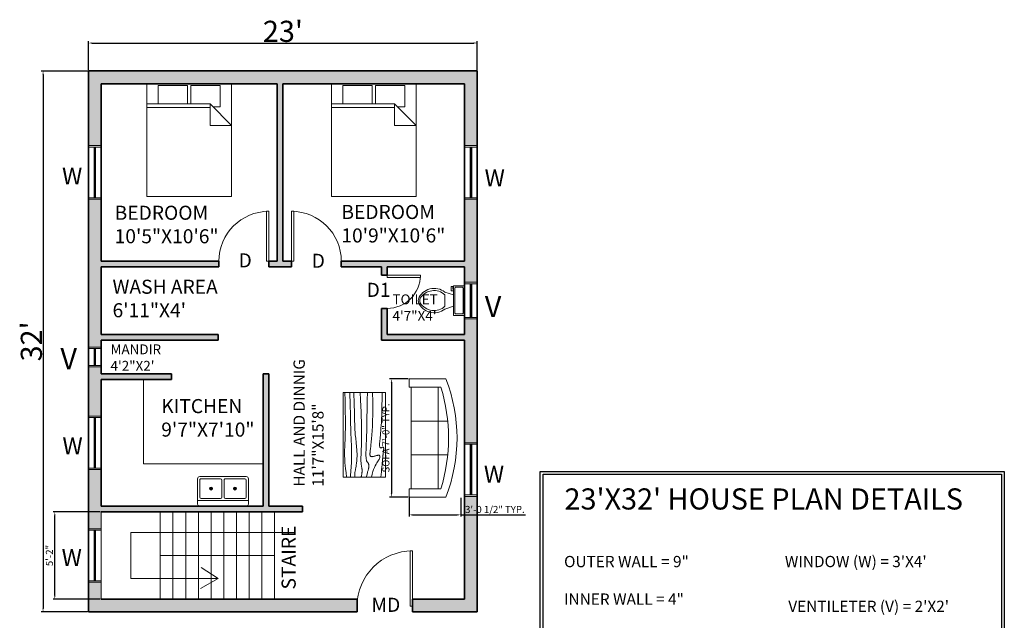
# Model space of a CAD drawing. Units: inches. Extents: x 1662 to 23131, y 1265 to 19127.
# Tile 7 of 26: x 12445 to 13143, y 5870 to 6296. Entities that reach past the tile are written whole.
import ezdxf

# ---------------------------------------------------------------- set-up
doc = ezdxf.new("R2010")
doc.units = ezdxf.units.IN
for name, color, linetype, lineweight in [('A-ANNO-DIMS', 4, 'Continuous', 18), ('A-ANNO-IDEN', 7, 'Continuous', 18), ('A-ANNO-TEXT', 7, 'Continuous', 18), ('A-ANNO-TITL', 7, 'Continuous', 35), ('A-ANNO-TTLB', 7, 'Continuous', 25), ('A-AREA-IDEN', 7, 'Continuous', 18), ('A-DOOR', 3, 'Continuous', 18), ('A-FLOR-CASE', 8, 'Continuous', 18), ('A-FLOR-FIXT', 9, 'Continuous', 18), ('A-FLOR-STRS', 7, 'Continuous', 18), ('A-FURN', 8, 'Continuous', 18), ('A-GLAZ', 4, 'Continuous', 18), ('A-WALL', 7, 'Continuous', 35), ('A-WALL-PATT', 8, 'Continuous', 13)]:
    doc.layers.add(name, color=color, linetype=linetype, lineweight=lineweight)
doc.styles.get("Standard").update_dxf_attribs({"font": 'arial.ttf'})
doc.dimstyles.new('ISO-25', dxfattribs={"dimtxt": 5, "dimasz": 2.5, "dimexe": 1.25, "dimexo": 0.625, "dimtad": 1, "dimlunit": 3, "dimtxsty": 'Standard', "dimcen": 2.5, "dimadec": 0, "dimazin": 0, "dimtfac": 1, "dimtmove": 0, "dimatfit": 3, "dimfxl": 1, "dimarcsym": 0})

# ---------------------------------------------------------------- blocks, each defined once
blk = doc.blocks.new('*U51')
for p, q in [((0, 0), (0, -100)), ((-1000, 0), (-1000, -100))]:
    blk.add_line(p, q)
blk.add_lwpolyline([(0, 0), (0, 1000), (-43.75, 1000), (-43.75, 0)], close=True)
blk.add_arc((0, 0), 1000, 90, 180)
blk = doc.blocks.new('*U26')
for p, q in [((0, 0), (0, -100)), ((900, 0), (900, -100))]:
    blk.add_line(p, q)
blk.add_lwpolyline([(0, 0), (0, 900), (43.75, 900), (43.75, 0)], close=True)
blk.add_arc((0, 0), 900, 0, 90)
blk = doc.blocks.new('*U4')
for p, q in [((0, 0), (0, -100)), ((-900, 0), (-900, -100))]:
    blk.add_line(p, q)
blk.add_lwpolyline([(0, 0), (0, 900), (-43.75, 900), (-43.75, 0)], close=True)
blk.add_arc((0, 0), 900, 90, 180)
blk = doc.blocks.new('*U28')
for p, q in [((0, 0), (0, -100)), ((600, 0), (600, -100))]:
    blk.add_line(p, q)
blk.add_lwpolyline([(0, 0), (0, 600), (43.75, 600), (43.75, 0)], close=True)
blk.add_arc((0, 0), 600, 0, 90)
blk = doc.blocks.new('Bed - Queen')
for p, q in [((0, -80.00003), (0, 0)), ((0, 0), (59.99999, 0)), ((59.99999, 0), (59.99999, -80.00003)), ((7.99999, -1.2), (28.79998, -1.2)), ((7.99999, -14.4), (7.99999, -1.2)), ((28.79998, -1.2), (28.79998, -14.4)), ((31.19999, -1.2), (51.99999, -1.2)), ((31.19999, -14.4), (31.19999, -1.2)), ((51.99999, -1.2), (51.99999, -16.4)), ((0, -14.4), (44.8, -14.4)), ((44.8, -16.8), (0, -16.8)), ((59.99999, -29.6), (44.8, -14.4)), ((44.8, -14.4), (44.8, -29.6)), ((51.99999, -16.4), (46.79936, -16.4)), ((44.8, -29.6), (59.99999, -29.6)), ((59.99999, -80.00003), (0, -80.00003))]:
    blk.add_line(p, q)
blk = doc.blocks.new('Sink-double - 36 in top')
for p, q in [((-18, -4), (18, -4)), ((-0.75, -18.5), (-0.75, -6.5)), ((0.75, -6.5), (0.75, -18.5))]:
    blk.add_line(p, q)
for points in [[(-16.5, 0), (16.5, 0)], [(-18, -19.5), (-18, -1.5)], [(-16.5, -18.5), (-16.5, -6.5)], [(-15.5, -5.5), (-1.75, -5.5)], [(1.75, -5.5), (15.5, -5.5)], [(16.5, -6.5), (16.5, -18.5)], [(18, -1.5), (18, -19.5)], [(-1.75, -19.5), (-15.5, -19.5)], [(15.5, -19.5), (1.75, -19.5)], [(16.5, -21), (-16.5, -21)]]:
    blk.add_lwpolyline(points)
for centre, radius in [((-8.5, -12.5), 1), ((-8.5, -12.5), 0.5), ((8.5, -12.5), 1), ((8.5, -12.5), 0.5)]:
    blk.add_circle(centre, radius)
for centre, radius, start, end in [((-16.5, -1.5), 1.5, 90, 180), ((16.5, -1.5), 1.5, 0, 90), ((-15.5, -6.5), 1, 90, 180), ((-1.75, -6.5), 1, 0, 90), ((1.75, -6.5), 1, 90, 180), ((15.5, -6.5), 1, 0, 90), ((-16.5, -19.5), 1.5, 180, 270), ((-15.5, -18.5), 1, 180, 270), ((-1.75, -18.5), 1, 270, 0), ((1.75, -18.5), 1, 180, 270), ((15.5, -18.5), 1, 270, 0), ((16.5, -19.5), 1.5, 270, 0)]:
    blk.add_arc(centre, radius, start, end)
blk = doc.blocks.new('Toilet - top')
for p, q in [((9.5, -6), (9.5, -2)), ((-10, -8.5), (-8, -8.5)), ((-10, -9.5), (-10, -8.5)), ((-7, -9.5), (-10, -9.5)), ((-8, -8.5), (-8, -8)), ((-7, -8), (-7, -9.5)), ((-4, -8), (-6, -14)), ((4, -8), (6, -14)), ((4, -14), (-4, -14))]:
    blk.add_line(p, q)
blk.add_lwpolyline([(10.5, -8), (10.5, 0), (-10.5, 0), (-10.5, -8)], close=True)
for points in [[(-9.5, -2), (-9.5, -6)], [(8.5, -1), (-8.5, -1)], [(-8.5, -7), (8.5, -7)]]:
    blk.add_lwpolyline(points)
for centre, radius, start, end in [((-8.62, -1.88), 0.884, 81.8699, 188.1301), ((-8.62, -6.12), 0.884, 171.8699, 278.1301), ((8.62, -1.88), 0.884, 351.8699, 98.1301), ((8.62, -6.12), 0.884, 261.8699, 8.1301), ((3.52, -21.58), 12.17, 141.46911, 247.97143), ((4.2, -21.82), 11.33, 136.36773, 238.94682), ((-3.52, -21.58), 12.17, 292.02843, 38.53071), ((-4.2, -21.82), 11.33, 301.05301, 43.63209), ((0, -27.88), 4, 245.73182, 294.26817), ((0, -29), 4, 254.86053, 285.13947)]:
    blk.add_arc(centre, radius, start, end)
blk = doc.blocks.new('Table - Rectangular Woodgrain 60 x 30 in.')
for p, q in [((0, 0), (0, -30)), ((60, 0), (0, 0)), ((60, -30), (60, 0)), ((0, -30), (60, -30))]:
    blk.add_line(p, q)
for points in [[(0, -2.4), (4.8155, -2.418), (9.0302, -2.4688), (12.709, -2.5477), (15.9167, -2.65), (18.7181, -2.7711), (21.1781, -2.9063), (23.3616, -3.0508), (25.3333, -3.2), (27.1477, -3.3495), (28.8172, -3.4958), (30.3437, -3.636), (31.7291, -3.7667), (32.9756, -3.8849), (34.0849, -3.9875), (35.059, -4.0714), (35.9, -4.1334), (36.6114, -4.1711), (37.2041, -4.1854), (37.6906, -4.1779), (38.0833, -4.15), (38.3948, -4.1034), (38.6375, -4.0396), (38.8239, -3.9602), (38.9666, -3.8667), (39.0764, -3.7608), (39.1573, -3.6448), (39.2116, -3.521), (39.2416, -3.3917), (39.2498, -3.2593), (39.2385, -3.1261), (39.21, -2.9944), (39.1666, -2.8667), (39.111, -2.7447), (39.0468, -2.6281), (38.978, -2.5163), (38.9083, -2.4083), (38.8418, -2.3035), (38.7823, -2.201), (38.7337, -2.1001), (38.7, -2), (38.6844, -1.9003), (38.6875, -1.8021), (38.7094, -1.707), (38.75, -1.6167), (38.8094, -1.5326), (38.8875, -1.4563), (38.9844, -1.3893), (39.1, -1.3333), (39.2351, -1.2896), (39.3937, -1.2583), (39.5804, -1.2396), (39.8, -1.2333), (40.057, -1.2396), (40.3562, -1.2583), (40.7023, -1.2896), (41.1, -1.3333), (41.5547, -1.3895), (42.0755, -1.4573), (42.6721, -1.5361), (43.3542, -1.625), (44.1316, -1.7233), (45.014, -1.8302), (46.0114, -1.9449), (47.1333, -2.0667), (48.3862, -2.1947), (49.7625, -2.3281), (51.2513, -2.4663), (52.8416, -2.6083), (54.5226, -2.7535), (56.2833, -2.9011), (58.1127, -3.0501), (60, -3.2)], [(0, -9.2), (6.5759, -9.0858), (11.9385, -9.0365), (16.2527, -9.0418), (19.6833, -9.0917), (22.3952, -9.1759), (24.5531, -9.2844), (26.322, -9.4069), (27.8666, -9.5333), (29.3241, -9.6553), (30.7203, -9.7719), (32.0532, -9.8837), (33.3208, -9.9917), (34.5213, -10.0965), (35.6526, -10.199), (36.7128, -10.2999), (37.7, -10.4), (38.6129, -10.4996), (39.4531, -10.5969), (40.223, -10.6895), (40.925, -10.775), (41.5613, -10.8512), (42.1344, -10.9156), (42.6465, -10.966), (43.1, -11), (43.4976, -11.0158), (43.8437, -11.0136), (44.143, -10.9942), (44.4, -10.9583), (44.6195, -10.9069), (44.8062, -10.8406), (44.9648, -10.7603), (45.1, -10.6667), (45.2155, -10.5598), (45.3114, -10.4365), (45.3871, -10.2929), (45.4416, -10.125), (45.4743, -9.929), (45.4844, -9.7011), (45.4709, -9.4371), (45.4333, -9.1333), (45.3716, -8.7883), (45.2896, -8.4104), (45.1919, -8.0107), (45.0833, -7.6), (44.9685, -7.1893), (44.8521, -6.7896), (44.7388, -6.4117), (44.6333, -6.0667), (44.54, -5.7628), (44.4614, -5.4979), (44.4001, -5.2675), (44.3583, -5.0667), (44.3384, -4.8909), (44.3427, -4.7354), (44.3736, -4.5956), (44.4333, -4.4667), (44.5236, -4.3453), (44.6427, -4.2333), (44.7884, -4.1339), (44.9583, -4.05), (45.1501, -3.9849), (45.3614, -3.9417), (45.59, -3.9234), (45.8333, -3.9333), (46.0915, -3.9749), (46.3734, -4.0531), (46.6906, -4.1736), (47.0542, -4.3417), (47.4756, -4.5629), (47.9661, -4.8427), (48.5372, -5.1866), (49.2, -5.6), (49.9676, -6.0844), (50.8594, -6.625), (51.8965, -7.2031), (53.1, -7.8), (54.491, -8.3969), (56.0906, -8.975), (57.9199, -9.5156), (60, -10)], [(0, -12.8), (5.1847, -12.9322), (9.6213, -13.0323), (13.3963, -13.1059), (16.5958, -13.1583), (19.3063, -13.1952), (21.614, -13.2219), (23.6054, -13.2439), (25.3666, -13.2667), (26.9728, -13.2947), (28.4531, -13.3281), (29.8256, -13.3663), (31.1083, -13.4083), (32.3191, -13.4535), (33.476, -13.501), (34.597, -13.5501), (35.7, -13.6), (36.7984, -13.6497), (37.8875, -13.6979), (38.9578, -13.743), (40, -13.7833), (41.0047, -13.8174), (41.9625, -13.8438), (42.864, -13.8607), (43.7, -13.8667), (44.4631, -13.8604), (45.1552, -13.8417), (45.7801, -13.8104), (46.3416, -13.7667), (46.8439, -13.7104), (47.2906, -13.6417), (47.6858, -13.5604), (48.0333, -13.4667), (48.3375, -13.3608), (48.6042, -13.2448), (48.8396, -13.121), (49.05, -12.9917), (49.2417, -12.8593), (49.4208, -12.7261), (49.5937, -12.5944), (49.7667, -12.4667), (49.9452, -12.3451), (50.1323, -12.2313), (50.3303, -12.1268), (50.5416, -12.0333), (50.7686, -11.9524), (51.0135, -11.8854), (51.2788, -11.8341), (51.5666, -11.8), (51.8785, -11.7843), (52.2116, -11.7865), (52.562, -11.8059), (52.926, -11.8417), (53.2998, -11.8931), (53.6795, -11.9594), (54.0614, -12.0397), (54.4416, -12.1333), (54.8223, -12.2401), (55.2293, -12.3625), (55.6942, -12.5037), (56.2489, -12.6667), (56.9251, -12.8547), (57.7545, -13.0708), (58.7689, -13.3182), (60, -13.6)], [(0, -18), (5.124, -17.7273), (9.6609, -17.5057), (13.6705, -17.3303), (17.2125, -17.1958), (20.3467, -17.0973), (23.1328, -17.0297), (25.6307, -16.9878), (27.9, -16.9667), (29.9928, -16.9617), (31.9302, -16.9703), (33.7254, -16.9907), (35.3917, -17.0208), (36.9423, -17.0588), (38.3906, -17.1026), (39.7499, -17.1503), (41.0333, -17.2), (42.2519, -17.2496), (43.4073, -17.2969), (44.4986, -17.3395), (45.525, -17.375), (46.4858, -17.4012), (47.3802, -17.4156), (48.2074, -17.416), (48.9667, -17.4), (49.6583, -17.3662), (50.2872, -17.3167), (50.8595, -17.2547), (51.3812, -17.1833), (51.8584, -17.1057), (52.2971, -17.025), (52.7034, -16.9443), (53.0833, -16.8667), (53.443, -16.7951), (53.789, -16.7313), (54.128, -16.6768), (54.4666, -16.6334), (54.8115, -16.6024), (55.1693, -16.5854), (55.5465, -16.5841), (55.95, -16.6), (56.3828, -16.6337), (56.8346, -16.6823), (57.2915, -16.7418), (57.7396, -16.8084), (58.165, -16.878), (58.5539, -16.9469), (58.8924, -17.0111), (59.1666, -17.0667), (59.3679, -17.1107), (59.5078, -17.1438), (59.6032, -17.1675), (59.6708, -17.1833), (59.7275, -17.193), (59.7901, -17.1979), (59.8753, -17.1998), (60, -17.2)], [(0, -22.4), (8.0098, -22.2501), (14.4094, -22.1011), (19.4168, -21.9535), (23.25, -21.8083), (26.1269, -21.6663), (28.2656, -21.5281), (29.884, -21.3947), (31.2, -21.2667), (32.3967, -21.1448), (33.5172, -21.0292), (34.5697, -20.9198), (35.5625, -20.8167), (36.5037, -20.7198), (37.4015, -20.6292), (38.2642, -20.5448), (39.1, -20.4667), (39.9164, -20.3951), (40.7187, -20.3313), (41.5117, -20.2768), (42.3, -20.2333), (43.0883, -20.2024), (43.8812, -20.1854), (44.6836, -20.1841), (45.5, -20.2), (46.3328, -20.234), (47.1747, -20.2844), (48.0163, -20.3488), (48.8479, -20.425), (49.66, -20.5106), (50.4429, -20.6031), (51.1872, -20.7004), (51.8833, -20.8), (52.5246, -20.8999), (53.1166, -20.9995), (53.6681, -21.0983), (54.1875, -21.1958), (54.6834, -21.2919), (55.1646, -21.3859), (55.6394, -21.4777), (56.1167, -21.5667), (56.6028, -21.6515), (57.0961, -21.7266), (57.5929, -21.7852), (58.0896, -21.8208), (58.5823, -21.8268), (59.0674, -21.7964), (59.5412, -21.723), (60, -21.6)], [(0, -25.2), (8.6355, -25.0504), (15.7026, -24.9031), (21.4049, -24.7606), (25.9458, -24.625), (29.529, -24.4988), (32.3578, -24.3844), (34.6359, -24.284), (36.5667, -24.2), (38.3213, -24.1341), (39.9417, -24.0854), (41.437, -24.0523), (42.8167, -24.0333), (44.0901, -24.0268), (45.2667, -24.0313), (46.3557, -24.0451), (47.3667, -24.0667), (48.309, -24.0947), (49.1928, -24.1287), (50.0284, -24.168), (50.826, -24.2125), (51.5959, -24.2617), (52.3483, -24.3151), (53.0935, -24.3725), (53.8417, -24.4334), (54.6009, -24.497), (55.3699, -24.561), (56.1454, -24.6226), (56.9239, -24.6792), (57.7021, -24.7279), (58.4764, -24.7662), (59.2435, -24.7911), (60, -24.8)], [(0, -28.8), (5.6867, -28.6681), (10.45, -28.5698), (14.407, -28.5012), (17.675, -28.4584), (20.3711, -28.4374), (22.6125, -28.4344), (24.5164, -28.4455), (26.2, -28.4667), (27.762, -28.4947), (29.2276, -28.5281), (30.6033, -28.5663), (31.8958, -28.6084), (33.1118, -28.6535), (34.2578, -28.7011), (35.3405, -28.7501), (36.3666, -28.8), (37.3443, -28.8497), (38.288, -28.8974), (39.2137, -28.9412), (40.1375, -28.9792), (41.0753, -29.0093), (42.0432, -29.0297), (43.0572, -29.0384), (44.1333, -29.0333), (45.2936, -29.0114), (46.5843, -28.9641), (48.0579, -28.8816), (49.7666, -28.7542), (51.7629, -28.5721), (54.0989, -28.3255), (56.8272, -28.0048), (60, -27.6)]]:
    blk.add_lwpolyline(points)
blk = doc.blocks.new('Sofa - Roundback 7 ft.')
for p, q in [((-12.00002, -32.4421), (-12.00003, -6.5971)), ((11.99997, -32.4421), (11.99998, -6.5971)), ((-36.000027, -34), (-36.000027, -11.4696)), ((-35.999844, -13.3819), (35.9998, -13.3819)), ((35.99998, -34), (35.99998, -11.4696)), ((-36.000027, -32.4421), (35.99998, -32.4421))]:
    blk.add_line(p, q)
for points in [[(-36.000027, -34), (-42.000027, -34), (-42.000027, -8)], [(41.99998, -8), (41.99998, -34), (35.99998, -34)]]:
    blk.add_lwpolyline(points)
for centre, radius, start, end in [((0, -114.25), 114.25, 68.43141, 111.5686), ((-0.00001, -127.1968), 121.1968, 72.72033, 107.2797)]:
    blk.add_arc(centre, radius, start, end)
blk = doc.blocks.new('*D54')
at = {"layer": 'A-ANNO-DIMS', "color": 0, "lineweight": -2, "transparency": 16777216}
for p, q in [((12493.33, 6260.67), (12493.33, 6281.16)), ((12495.83, 6279.91), (12766.83, 6279.91)), ((12769.33, 6260.67), (12769.33, 6281.16))]:
    blk.add_line(p, q, dxfattribs=at)
at = {"layer": 'A-ANNO-DIMS', "color": 0, "transparency": 16777216}
for points in [[(12495.83, 6280.32), (12495.83, 6279.49), (12493.33, 6279.91)], [(12766.83, 6280.32), (12766.83, 6279.49), (12769.33, 6279.91)]]:
    blk.add_solid(points, dxfattribs=at)
at = {"layer": 'Defpoints', "color": 0, "transparency": 16777216}
for p in [(12769.33, 6279.91), (12493.33, 6260.04), (12769.33, 6260.04)]:
    blk.add_point(p, dxfattribs=at)
at = {"layer": 'A-ANNO-DIMS', "color": 0, "transparency": 16777216, "insert": (12631.33, 6288.2), "char_height": 5, "attachment_point": 5}
blk.add_mtext("{\\H3x;23'}", dxfattribs=at)
blk = doc.blocks.new('*D55')
at = {"layer": 'A-ANNO-DIMS', "color": 0, "lineweight": -2, "transparency": 16777216}
for p, q in [((12492.7, 6260.04), (12459.84, 6260.04)), ((12461.09, 6257.54), (12461.09, 5878.54)), ((12492.7, 5876.04), (12459.84, 5876.04))]:
    blk.add_line(p, q, dxfattribs=at)
at = {"layer": 'A-ANNO-DIMS', "color": 0, "transparency": 16777216}
for points in [[(12460.68, 6257.54), (12461.51, 6257.54), (12461.09, 6260.04)], [(12460.68, 5878.54), (12461.51, 5878.54), (12461.09, 5876.04)]]:
    blk.add_solid(points, dxfattribs=at)
at = {"layer": 'Defpoints', "color": 0, "transparency": 16777216}
for p in [(12493.33, 6260.04), (12461.09, 5876.04), (12493.33, 5876.04)]:
    blk.add_point(p, dxfattribs=at)
at = {"layer": 'A-ANNO-DIMS', "color": 0, "transparency": 16777216, "insert": (12452.8, 6068.04), "char_height": 5, "attachment_point": 5, "rotation": 90}
blk.add_mtext("{\\H3x;32'}", dxfattribs=at)
blk = doc.blocks.new('*D165')
at = {"layer": 'A-ANNO-DIMS', "color": 0, "lineweight": -2, "transparency": 16777216}
for p, q in [((12720.3, 6041.5), (12707.07, 6041.5)), ((12708.32, 6039), (12708.32, 5960)), ((12720.3, 5957.5), (12707.07, 5957.5))]:
    blk.add_line(p, q, dxfattribs=at)
at = {"layer": 'A-ANNO-DIMS', "color": 0, "transparency": 16777216}
for points in [[(12707.9, 6039), (12708.74, 6039), (12708.32, 6041.5)], [(12707.9, 5960), (12708.74, 5960), (12708.32, 5957.5)]]:
    blk.add_solid(points, dxfattribs=at)
at = {"layer": 'Defpoints', "color": 0, "transparency": 16777216}
for p in [(12720.92, 6041.5), (12708.32, 5957.5), (12720.92, 5957.5)]:
    blk.add_point(p, dxfattribs=at)
at = {"layer": 'A-ANNO-DIMS', "color": 0, "transparency": 16777216, "insert": (12705.11, 5999.5), "char_height": 5, "attachment_point": 5, "rotation": 90}
blk.add_mtext('SOFA 7\'-0" TYP.', dxfattribs=at)
blk = doc.blocks.new('*D166')
at = {"layer": 'A-ANNO-DIMS', "color": 0, "lineweight": -2, "transparency": 16777216}
for p, q in [((12720.92, 5956.88), (12720.92, 5943.65)), ((12757.59, 5956.88), (12757.59, 5943.65)), ((12723.42, 5944.9), (12755.09, 5944.9)), ((12757.59, 5944.9), (12803.46, 5944.9))]:
    blk.add_line(p, q, dxfattribs=at)
at = {"layer": 'A-ANNO-DIMS', "color": 0, "transparency": 16777216}
for points in [[(12723.42, 5945.32), (12723.42, 5944.48), (12720.92, 5944.9)], [(12755.09, 5945.32), (12755.09, 5944.48), (12757.59, 5944.9)]]:
    blk.add_solid(points, dxfattribs=at)
at = {"layer": 'Defpoints', "color": 0, "transparency": 16777216}
for p in [(12720.92, 5957.5), (12757.59, 5957.5), (12757.59, 5944.9)]:
    blk.add_point(p, dxfattribs=at)
at = {"layer": 'A-ANNO-DIMS', "color": 0, "transparency": 16777216, "insert": (12781.78, 5948.11), "char_height": 5, "attachment_point": 5}
blk.add_mtext('3\'-0 1/2" TYP.', dxfattribs=at)
blk = doc.blocks.new('*D219')
at = {"layer": 'A-ANNO-DIMS', "color": 0, "lineweight": -2, "transparency": 16777216}
for p, q in [((12501.7, 5947.04), (12468.18, 5947.04)), ((12469.43, 5887.54), (12469.43, 5944.54)), ((12501.7, 5885.04), (12468.18, 5885.04))]:
    blk.add_line(p, q, dxfattribs=at)
at = {"layer": 'A-ANNO-DIMS', "color": 0, "transparency": 16777216}
for points in [[(12469.01, 5944.54), (12469.85, 5944.54), (12469.43, 5947.04)], [(12469.01, 5887.54), (12469.85, 5887.54), (12469.43, 5885.04)]]:
    blk.add_solid(points, dxfattribs=at)
at = {"layer": 'Defpoints', "color": 0, "transparency": 16777216}
for p in [(12469.43, 5947.04), (12502.33, 5947.04), (12502.33, 5885.04)]:
    blk.add_point(p, dxfattribs=at)
at = {"layer": 'A-ANNO-DIMS', "color": 0, "transparency": 16777216, "insert": (12466.25, 5916.04), "char_height": 5, "attachment_point": 5, "rotation": 90}
blk.add_mtext('5\'-2"', dxfattribs=at)

msp = doc.modelspace()

# ---------------------------------------------------------------- hatches: boundary and pattern name
at = {"layer": 'A-WALL-PATT'}
h = msp.add_hatch(color=256, dxfattribs=at)
h.dxf.hatch_style = 1
h.paths.add_polyline_path([(12502.33, 6251.044), (12627.33, 6251.044), (12627.33, 6125.044), (12621.33, 6125.044), (12621.33, 6121.044), (12637.33, 6121.044), (12637.33, 6125.044), (12631.33, 6125.044), (12631.33, 6251.044), (12760.33, 6251.044), (12760.33, 6207.044), (12769.33, 6207.044), (12769.33, 6260.044), (12493.33, 6260.044), (12493.33, 6207.044), (12502.33, 6207.044)])
h.paths.add_polyline_path([(12769.33, 6169.044), (12760.33, 6169.044), (12760.33, 6125.044), (12672.763, 6125.044), (12672.763, 6121.044), (12701.33, 6121.044), (12701.33, 6115.044), (12705.33, 6115.044), (12705.33, 6121.044), (12760.33, 6121.044), (12760.33, 6110.044), (12769.33, 6110.044)])
h.paths.add_polyline_path([(12502.33, 6169.044), (12493.33, 6169.044), (12493.33, 6064.044), (12502.33, 6064.044), (12502.33, 6069.044), (12552.33, 6069.044), (12585.33, 6069.044), (12585.33, 6073.044), (12502.33, 6073.044), (12502.33, 6121.044), (12585.897, 6121.044), (12585.897, 6125.044), (12502.33, 6125.044)])
h.paths.add_polyline_path([(12502.33, 5977.044), (12493.33, 5977.044), (12493.33, 5935.044), (12502.33, 5935.044), (12502.33, 5947.044), (12645.33, 5947.044), (12645.33, 5951.044), (12621.33, 5951.044), (12621.33, 6045.044), (12617.33, 6045.044), (12617.33, 5951.044), (12502.33, 5951.044)])
h.paths.add_polyline_path([(12502.33, 6041.044), (12552.33, 6041.044), (12552.33, 6045.044), (12502.33, 6045.044), (12502.33, 6050.044), (12493.33, 6050.044), (12493.33, 6015.044), (12502.33, 6015.044)])
h.paths.add_polyline_path([(12683.96, 5885.044), (12645.33, 5885.044), (12502.33, 5885.044), (12502.33, 5897.044), (12493.33, 5897.044), (12493.33, 5876.044), (12683.96, 5876.044), (12683.96, 5879.981)])
h.paths.add_polyline_path([(12769.33, 5958.044), (12760.33, 5958.044), (12760.33, 5885.044), (12723.33, 5885.044), (12723.33, 5879.981), (12723.33, 5876.044), (12769.33, 5876.044)])
h.paths.add_polyline_path([(12769.33, 6084.044), (12760.33, 6084.044), (12760.33, 6073.044), (12705.33, 6073.044), (12705.33, 6091.422), (12701.33, 6091.422), (12701.33, 6069.044), (12760.33, 6069.044), (12760.33, 5996.044), (12769.33, 5996.044)])

# ---------------------------------------------------------------- linework, layer by layer
at = {"layer": 'A-ANNO-TTLB'}
for points in [[(12814.019, 5975.699), (13143.349, 5975.699), (13143.349, 5791.544), (12814.019, 5791.544)], [(12816.019, 5973.699), (13141.349, 5973.699), (13141.349, 5793.544), (12816.019, 5793.544)]]:
    msp.add_lwpolyline(points, close=True, dxfattribs=at)
at = {"layer": 'A-FLOR-CASE'}
for p, q in [((12532.33, 6041.044), (12532.33, 5981.044)), ((12532.33, 5981.044), (12617.33, 5981.044))]:
    msp.add_line(p, q, dxfattribs=at)
at = {"layer": 'A-FLOR-STRS'}
for p, q in [((12502.33, 5947.044), (12502.33, 5885.044)), ((12544.33, 5947.044), (12544.33, 5885.044)), ((12553.33, 5947.044), (12553.33, 5885.044)), ((12562.33, 5947.044), (12562.33, 5885.044)), ((12571.33, 5947.044), (12571.33, 5885.044)), ((12580.33, 5947.044), (12580.33, 5885.044)), ((12589.33, 5947.044), (12589.33, 5885.044)), ((12598.33, 5947.044), (12598.33, 5885.044)), ((12607.33, 5947.044), (12607.33, 5885.044)), ((12616.33, 5947.044), (12616.33, 5885.044)), ((12625.33, 5947.044), (12625.33, 5885.044)), ((12640.171, 5932.439), (12523.514, 5932.439)), ((12523.514, 5932.439), (12523.514, 5899.704)), ((12544.33, 5916.044), (12625.33, 5916.044)), ((12585.352, 5899.704), (12573.255, 5907.53)), ((12523.514, 5899.704), (12585.352, 5899.704)), ((12585.352, 5899.704), (12572.775, 5892.569))]:
    msp.add_line(p, q, dxfattribs=at)
at = {"layer": 'A-GLAZ'}
for p, q in [((12502.33, 6207.044), (12493.33, 6207.044)), ((12502.33, 6206.044), (12493.33, 6206.044)), ((12497.33, 6206.044), (12497.33, 6170.044)), ((12497.83, 6206.044), (12497.83, 6170.044)), ((12498.33, 6206.044), (12498.33, 6170.044)), ((12769.33, 6207.044), (12760.33, 6207.044)), ((12769.33, 6206.044), (12760.33, 6206.044)), ((12764.33, 6206.044), (12764.33, 6170.044)), ((12764.83, 6206.044), (12764.83, 6170.044)), ((12765.33, 6206.044), (12765.33, 6170.044)), ((12502.33, 6170.044), (12493.33, 6170.044)), ((12502.33, 6169.044), (12493.33, 6169.044)), ((12769.33, 6170.044), (12760.33, 6170.044)), ((12769.33, 6169.044), (12760.33, 6169.044)), ((12769.33, 6110.044), (12760.33, 6110.044)), ((12769.33, 6109.044), (12760.33, 6109.044)), ((12764.33, 6109.044), (12764.33, 6085.044)), ((12764.83, 6109.044), (12764.83, 6085.044)), ((12765.33, 6109.044), (12765.33, 6085.044)), ((12769.33, 6085.044), (12760.33, 6085.044)), ((12769.33, 6084.044), (12760.33, 6084.044)), ((12502.33, 6064.044), (12493.33, 6064.044)), ((12502.33, 6063.044), (12493.33, 6063.044)), ((12497.33, 6063.044), (12497.33, 6051.044)), ((12497.83, 6063.044), (12497.83, 6051.044)), ((12498.33, 6063.044), (12498.33, 6051.044)), ((12502.33, 6051.044), (12493.33, 6051.044)), ((12502.33, 6050.044), (12493.33, 6050.044)), ((12502.33, 6015.044), (12493.33, 6015.044)), ((12502.33, 6014.044), (12493.33, 6014.044)), ((12497.33, 6014.044), (12497.33, 5978.044)), ((12497.83, 6014.044), (12497.83, 5978.044)), ((12498.33, 6014.044), (12498.33, 5978.044)), ((12769.33, 5996.044), (12760.33, 5996.044)), ((12769.33, 5995.044), (12760.33, 5995.044)), ((12764.33, 5995.044), (12764.33, 5959.044)), ((12764.83, 5995.044), (12764.83, 5959.044)), ((12765.33, 5995.044), (12765.33, 5959.044)), ((12502.33, 5978.044), (12493.33, 5978.044)), ((12502.33, 5977.044), (12493.33, 5977.044)), ((12769.33, 5959.044), (12760.33, 5959.044)), ((12769.33, 5958.044), (12760.33, 5958.044)), ((12502.33, 5935.044), (12493.33, 5935.044)), ((12502.33, 5934.044), (12493.33, 5934.044)), ((12497.33, 5934.044), (12497.33, 5898.044)), ((12497.83, 5934.044), (12497.83, 5898.044)), ((12498.33, 5934.044), (12498.33, 5898.044)), ((12502.33, 5898.044), (12493.33, 5898.044)), ((12502.33, 5897.044), (12493.33, 5897.044))]:
    msp.add_line(p, q, dxfattribs=at)
at = {"layer": 'A-WALL'}
for p, q in [((12493.33, 6260.044), (12769.33, 6260.044)), ((12493.33, 6260.044), (12493.33, 5876.044)), ((12769.33, 5876.044), (12769.33, 6260.044)), ((12502.33, 6251.044), (12502.33, 6125.044)), ((12502.33, 6251.044), (12627.33, 6251.044)), ((12627.33, 6251.044), (12627.33, 6125.044)), ((12631.33, 6251.044), (12631.33, 6125.044)), ((12631.33, 6251.044), (12760.33, 6251.044)), ((12760.33, 6125.044), (12760.33, 6251.044)), ((12502.33, 6125.044), (12585.897, 6125.044)), ((12585.897, 6125.044), (12585.897, 6121.044)), ((12621.33, 6125.044), (12621.33, 6121.044)), ((12621.33, 6125.044), (12627.33, 6125.044)), ((12631.33, 6125.044), (12637.33, 6125.044)), ((12637.33, 6125.044), (12637.33, 6121.044)), ((12672.763, 6125.044), (12672.763, 6121.044)), ((12672.763, 6125.044), (12760.33, 6125.044)), ((12502.33, 6121.044), (12585.33, 6121.044)), ((12502.33, 6121.044), (12585.897, 6121.044)), ((12502.33, 6121.044), (12502.33, 6073.044)), ((12621.33, 6121.044), (12637.33, 6121.044)), ((12672.763, 6121.044), (12701.33, 6121.044)), ((12701.33, 6115.044), (12701.33, 6121.044)), ((12701.33, 6115.044), (12705.33, 6115.044)), ((12705.33, 6121.044), (12760.33, 6121.044)), ((12705.33, 6115.044), (12705.33, 6121.044)), ((12760.33, 6073.044), (12760.33, 6121.044)), ((12701.33, 6069.044), (12701.33, 6091.422)), ((12701.33, 6091.422), (12705.33, 6091.422)), ((12705.33, 6073.044), (12705.33, 6091.422)), ((12502.33, 6073.044), (12585.33, 6073.044)), ((12585.33, 6073.044), (12585.33, 6069.044)), ((12705.33, 6073.044), (12760.33, 6073.044)), ((12502.33, 6069.044), (12552.33, 6069.044)), ((12502.33, 6069.044), (12502.33, 6045.044)), ((12552.33, 6069.044), (12585.33, 6069.044)), ((12701.33, 6069.044), (12760.33, 6069.044)), ((12760.33, 5885.044), (12760.33, 6069.044)), ((12502.33, 6045.044), (12552.33, 6045.044)), ((12552.33, 6045.044), (12552.33, 6041.044)), ((12617.33, 6045.044), (12617.33, 5951.044)), ((12617.33, 6045.044), (12621.33, 6045.044)), ((12621.33, 6045.044), (12621.33, 5951.044)), ((12502.33, 6041.044), (12552.33, 6041.044)), ((12502.33, 6041.044), (12502.33, 5951.044)), ((12502.33, 5951.044), (12617.33, 5951.044)), ((12502.33, 5947.044), (12645.33, 5947.044)), ((12621.33, 5951.044), (12645.33, 5951.044)), ((12645.33, 5951.044), (12645.33, 5947.044)), ((12502.33, 5885.044), (12683.96, 5885.044)), ((12645.33, 5885.044), (12683.96, 5885.044)), ((12683.96, 5885.044), (12683.96, 5876.044)), ((12723.33, 5885.044), (12723.33, 5876.044)), ((12723.33, 5885.044), (12760.33, 5885.044)), ((12493.33, 5876.044), (12683.96, 5876.044)), ((12723.33, 5876.044), (12769.33, 5876.044))]:
    msp.add_line(p, q, dxfattribs=at)

# ---------------------------------------------------------------- block references
at = {"layer": 'A-DOOR', "xscale": 0.0393700787401575, "yscale": 0.0393700787401575, "zscale": 0.0393700787401575}
for name, p in [('*U4', (12621.33, 6124.981)), ('*U26', (12637.33, 6124.981)), ('*U51', (12723.33, 5879.981))]:
    msp.add_blockref(name, p, dxfattribs=at)
at = {"layer": 'A-DOOR', "xscale": 0.0393700787401575, "yscale": 0.0393700787401575, "zscale": 0.0393700787401575, "rotation": 270}
msp.add_blockref('*U28', (12705.267, 6115.044), dxfattribs=at)
at = {"layer": 'A-FLOR-FIXT'}
for name, p, rotation in [('Toilet - top', (12760.33, 6097.044), 270), ('Sink-double - 36 in top', (12588.824, 5951.044), 180)]:
    msp.add_blockref(name, p, dxfattribs=dict(at, rotation=rotation))
at = {"layer": 'A-FURN'}
for p in [(12534.83, 6251.044), (12665.83, 6251.044)]:
    msp.add_blockref('Bed - Queen', p, dxfattribs=at)
for name, p, rotation in [('Sofa - Roundback 7 ft.', (12754.921, 5999.5), 269.9999999999999), ('Table - Rectangular Woodgrain 60 x 30 in.', (12704.139, 6031.704), 270)]:
    msp.add_blockref(name, p, dxfattribs=dict(at, rotation=rotation))

# ---------------------------------------------------------------- texts
at = {"layer": 'A-ANNO-IDEN', "attachment_point": 1}
for s, width, heights, insert, char_height in [('W', 471.52273, [28.462], (12474.576, 6191.484), 12), ('W', 471.52273, [28.462], (12774.502, 6190.175), 12), ('D', 1142.59551, [0], (12599.88, 6130.581), 10), ('D', 1142.59551, [0], (12651.775, 6130.297), 10), ('D1', 1142.59551, [20], (12690.771, 6109.646), 10), ('V', 1142.59551, [20], (12774.612, 6100.367), 15), ('V', 1142.59551, [20], (12473.412, 6063.335), 15), ('W', 471.52273, [28.462], (12474.868, 5999.895), 12), ('W', 471.52273, [28.462], (12773.967, 5979.845), 12), ('W', 471.52273, [28.462], (12474.286, 5920.649), 12), ('MD', 1142.59551, [0], (12694.191, 5886.04), 10)]:
    msp.add_mtext_dynamic_manual_height_columns(s, width=width, gutter_width=12.5, heights=heights, dxfattribs=dict(at, insert=insert, char_height=char_height))
at = {"layer": 'A-ANNO-TEXT', "attachment_point": 1}
for s, heights, insert, char_height in [('OUTER WALL = 9"\\P\\PINNER WALL = 4"', [277.772], (12830.892, 5915.744), 8), ("{\\H0.8x;WINDOW (W) = 3'X4'}", [0], (12987.604, 5915.767), 10), ("{\\H0.8x; VENTILETER (V) = 2'X2'}", [0], (12987.604, 5883.957), 10)]:
    msp.add_mtext_dynamic_manual_height_columns(s, width=1142.59551, gutter_width=12.5, heights=heights, dxfattribs=dict(at, insert=insert, char_height=char_height))
at = {"layer": 'A-ANNO-TITL', "insert": (12831.22, 5963.704), "char_height": 15, "attachment_point": 1}
msp.add_mtext_dynamic_manual_height_columns("23'X32' HOUSE PLAN DETAILS", width=1142.59551, gutter_width=12.5, heights=[0], dxfattribs=at)
at = {"layer": 'A-AREA-IDEN', "attachment_point": 1}
for s, insert, char_height in [('BEDROOM\\P10\'5"X10\'6"', (12511.912, 6164.389), 10), ('BEDROOM\\P10\'9"X10\'6"', (12672.837, 6164.951), 10), ('WASH AREA\\P6\'11"X4\'', (12510.429, 6111.858), 10), ('TOILET\\P4\'7"X4\'', (12709.129, 6101.418), 7), ('MANDIR\\P4\'2"X2\'', (12508.991, 6065.898), 7), ('KITCHEN\\P9\'7"X7\'10"', (12544.987, 6027.112), 10)]:
    msp.add_mtext_dynamic_manual_height_columns(s, width=1142.59551, gutter_width=12.5, heights=[277.772], dxfattribs=dict(at, insert=insert, char_height=char_height))
at = {"layer": 'A-AREA-IDEN', "attachment_point": 1, "rotation": 90}
for s, heights, insert, char_height in [('HALL AND DINNIG\\P11\'7"X15\'8"', [277.772], (12638.869, 5964.943), 8), ('STAIRE ', [0], (12630.406, 5891.913), 10)]:
    msp.add_mtext_dynamic_manual_height_columns(s, width=1142.59551, gutter_width=12.5, heights=heights, dxfattribs=dict(at, insert=insert, char_height=char_height))

# ---------------------------------------------------------------- dimensions: what is measured, and where the dimension line sits
at = {"layer": 'A-ANNO-DIMS'}
for base, p1, p2, text, override, picture, middle in [((12769.33, 6279.907), (12493.33, 6260.044), (12769.33, 6260.044), '{\\H3x;<>}', {"dimclrd": 0, "dimclre": 0, "dimclrt": 0}, '*D54', (12631.33, 6288.195)), ((12757.588, 5944.9), (12720.921, 5957.5), (12757.588, 5957.5), '<> TYP.', {"dimdec": 1, "dimlfac": 1, "dimrnd": 0, "dimzin": 1, "dimdsep": 46, "dimlunit": 4, "dimfrac": 2}, '*D166', (12781.775, 5948.112))]:
    dim = msp.add_linear_dim(base=base, p1=p1, p2=p2, text=text, dimstyle='ISO-25', override=override, dxfattribs=at)
    dim.commit()
    dim.dimension.update_dxf_attribs({"geometry": picture, "text_midpoint": middle})
for base, p1, p2, angle, text, override, picture, middle in [((12461.093, 5876.044), (12493.33, 6260.044), (12493.33, 5876.044), 90, '{\\H3x;<>}', {"dimclrd": 0, "dimclre": 0, "dimclrt": 0}, '*D55', (12452.804, 6068.044)), ((12708.321, 5957.5), (12720.921, 6041.5), (12720.921, 5957.5), 270, 'SOFA <> TYP.', {"dimdec": 1, "dimlfac": 1, "dimrnd": 0, "dimzin": 1, "dimdsep": 46, "dimlunit": 4, "dimfrac": 2}, '*D165', (12705.109, 5999.5))]:
    dim = msp.add_linear_dim(base=base, p1=p1, p2=p2, angle=angle, text=text, dimstyle='ISO-25', override=override, dxfattribs=at)
    dim.commit()
    dim.dimension.update_dxf_attribs({"geometry": picture, "text_midpoint": middle})
dim = msp.add_linear_dim(base=(12469.43, 5947.044), p1=(12502.33, 5885.044), p2=(12502.33, 5947.044), angle=90, dimstyle='ISO-25', override={"dimdec": 1, "dimlfac": 1, "dimrnd": 0, "dimzin": 1, "dimdsep": 46, "dimlunit": 4, "dimfrac": 2}, dxfattribs=at)
dim.commit()
dim.dimension.update_dxf_attribs({"geometry": '*D219', "text_midpoint": (12466.252, 5916.044)})

doc.saveas('drawing.dxf')
